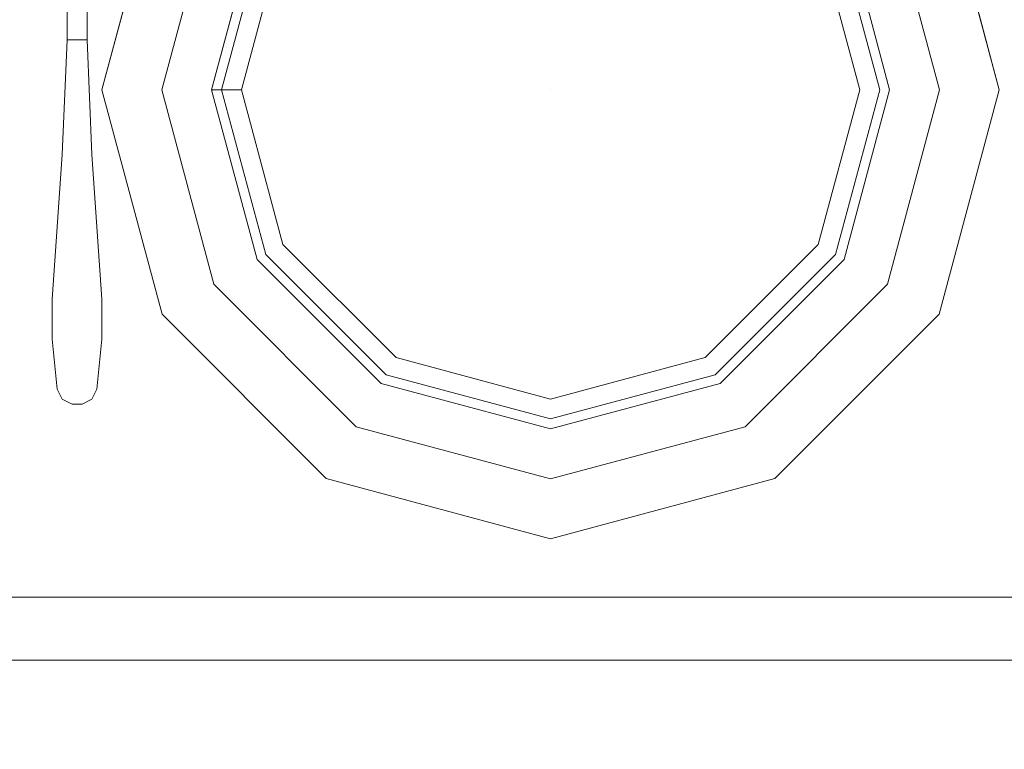
# Model space of a CAD drawing. Units: inches. Extents: x 375 to 1122, y 27 to 1069.
# Tile 86 of 155: x 719.12 to 731.28, y 845.63 to 854.63. Entities that reach past the tile are written whole.
import ezdxf

# ---------------------------------------------------------------- set-up
doc = ezdxf.new("R2010")
doc.units = ezdxf.units.IN
doc.layers.add('A-ANNO-DIMS', color=2, linetype='Continuous', lineweight=18)
doc.layers.add('Furniture', color=30, linetype='Continuous', lineweight=18)
doc.styles.get("Standard").update_dxf_attribs({"font": 'arial.ttf'})
doc.dimstyles.new('ISO-25', dxfattribs={"dimtxt": 12, "dimasz": 2.5, "dimexe": 1.5, "dimexo": 1.5, "dimtad": 1, "dimdec": 1, "dimlunit": 3, "dimtxsty": 'Standard', "dimblk": 'ARCHTICK', "dimcen": 2.5, "dimadec": 0, "dimazin": 0, "dimtfac": 1, "dimtdec": 1, "dimtmove": 0, "dimatfit": 3, "dimfxl": 1.5, "dimfxlon": 1, "dimarcsym": 0})

# ---------------------------------------------------------------- blocks, each defined once
blk = doc.blocks.new('A$C403C54AD')
for p, q in [((2.27071, 1.26108, -0.0006), (2.27071, 0.79569, -0.0006)), ((2.2901, 1.26108, -0.0006), (2.2901, 0.79569, -0.0006))]:
    blk.add_line(p, q)
at = {"linetype": 'ByBlock'}
for points, invisible_edges in [([(2.11411, 1.15687, -0.03783), (2.11411, 1.1384, -0.03783), (2.05409, 1.12232, -0.03783), (2.04485, 1.13831, -0.03783)], 5), ([(2.11411, 1.12301, -0.05168), (2.11411, 1.15687, -0.04244), (2.04485, 1.13831, -0.04244), (2.06178, 1.10899, -0.05168)], 5), ([(2.18338, 1.13831, -0.03783), (2.17414, 1.12232, -0.03783), (2.11411, 1.1384, -0.03783), (2.11411, 1.15687, -0.03783)], 5), ([(2.16645, 1.10899, -0.05168), (2.18338, 1.13831, -0.04244), (2.11411, 1.15687, -0.04244), (2.11411, 1.12301, -0.05168)], 5), ([(2.11411, 1.1384, -0.03783), (2.11411, 1.11993, -0.04398), (2.06332, 1.10632, -0.04398), (2.05409, 1.12232, -0.03783)], 5), ([(2.17414, 1.12232, -0.03783), (2.16491, 1.10632, -0.04398), (2.11411, 1.11993, -0.04398), (2.11411, 1.1384, -0.03783)], 5), ([(2.20476, 1.07068, -0.05168), (2.23408, 1.08761, -0.04244), (2.18338, 1.13831, -0.04244), (2.16645, 1.10899, -0.05168)], 5), ([(2.23408, 1.08761, -0.03783), (2.21809, 1.07837, -0.03783), (2.17414, 1.12232, -0.03783), (2.18338, 1.13831, -0.03783)], 5), ([(2.11411, 1.11377, -0.06091), (2.11411, 1.12301, -0.05168), (2.06178, 1.10899, -0.05168), (2.0664, 1.10099, -0.06091)], 5), ([(2.16183, 1.10099, -0.06091), (2.16645, 1.10899, -0.05168), (2.11411, 1.12301, -0.05168), (2.11411, 1.11377, -0.06091)], 5), ([(2.21809, 1.07837, -0.03783), (2.20209, 1.06914, -0.04398), (2.16491, 1.10632, -0.04398), (2.17414, 1.12232, -0.03783)], 5), ([(2.11411, 1.11993, -0.04398), (2.11411, 1.01834, -0.04398), (2.11411, 1.01834, -0.04398), (2.06332, 1.10632, -0.04398)], 5), ([(2.16491, 1.10632, -0.04398), (2.11411, 1.01834, -0.04398), (2.11411, 1.01834, -0.04398), (2.11411, 1.11993, -0.04398)], 5), ([(2.19676, 1.06606, -0.06091), (2.20476, 1.07068, -0.05168), (2.16645, 1.10899, -0.05168), (2.16183, 1.10099, -0.06091)], 5), ([(2.06332, 1.10632, -0.04398), (2.11411, 1.01834, -0.04398), (2.11411, 1.01834, -0.04398), (2.02614, 1.06914, -0.04398)], 5), ([(2.20209, 1.06914, -0.04398), (2.11411, 1.01834, -0.04398), (2.11411, 1.01834, -0.04398), (2.16491, 1.10632, -0.04398)], 5), ([(2.21878, 1.01834, -0.05168), (2.25264, 1.01834, -0.04244), (2.23408, 1.08761, -0.04244), (2.20476, 1.07068, -0.05168)], 5), ([(2.25264, 1.01834, -0.03783), (2.23417, 1.01834, -0.03783), (2.21809, 1.07837, -0.03783), (2.23408, 1.08761, -0.03783)], 5), ([(2.23417, 1.01834, -0.03783), (2.2157, 1.01834, -0.04398), (2.20209, 1.06914, -0.04398), (2.21809, 1.07837, -0.03783)], 5), ([(2.20954, 1.01834, -0.06091), (2.21878, 1.01834, -0.05168), (2.20476, 1.07068, -0.05168), (2.19676, 1.06606, -0.06091)], 5), ([(2.02614, 1.06914, -0.04398), (2.11411, 1.01834, -0.04398), (2.11411, 1.01834, -0.04398), (2.01253, 1.01834, -0.04398)], 5), ([(2.2157, 1.01834, -0.04398), (2.11411, 1.01834, -0.04398), (2.11411, 1.01834, -0.04398), (2.20209, 1.06914, -0.04398)], 5), ([(2.01253, 1.01834, -0.04398), (2.11411, 1.01834, -0.04398), (2.11411, 1.01834, -0.04398), (2.02614, 0.96755, -0.04398)], 5), ([(2.02614, 0.96755, -0.04398), (2.11411, 1.01834, -0.04398), (2.11411, 1.01834, -0.04398), (2.06332, 0.93037, -0.04398)], 5), ([(2.06332, 0.93037, -0.04398), (2.11411, 1.01834, -0.04398), (2.11411, 1.01834, -0.04398), (2.11411, 0.91676, -0.04398)], 5), ([(2.20209, 0.96755, -0.04398), (2.11411, 1.01834, -0.04398), (2.11411, 1.01834, -0.04398), (2.2157, 1.01834, -0.04398)], 5), ([(2.16491, 0.93037, -0.04398), (2.11411, 1.01834, -0.04398), (2.11411, 1.01834, -0.04398), (2.20209, 0.96755, -0.04398)], 5), ([(2.11411, 0.91676, -0.04398), (2.11411, 1.01834, -0.04398), (2.11411, 1.01834, -0.04398), (2.16491, 0.93037, -0.04398)], 5), ([(2.19676, 0.97063, -0.06091), (2.20476, 0.96601, -0.05168), (2.21878, 1.01834, -0.05168), (2.20954, 1.01834, -0.06091)], 5), ([(2.21809, 0.95832, -0.03783), (2.20209, 0.96755, -0.04398), (2.2157, 1.01834, -0.04398), (2.23417, 1.01834, -0.03783)], 5), ([(2.20476, 0.96601, -0.05168), (2.23408, 0.94908, -0.04244), (2.25264, 1.01834, -0.04244), (2.21878, 1.01834, -0.05168)], 5), ([(2.23408, 0.94908, -0.03783), (2.21809, 0.95832, -0.03783), (2.23417, 1.01834, -0.03783), (2.25264, 1.01834, -0.03783)], 5), ([(2.16183, 0.9357, -0.06091), (2.16645, 0.9277, -0.05168), (2.20476, 0.96601, -0.05168), (2.19676, 0.97063, -0.06091)], 5), ([(2.17414, 0.91437, -0.03783), (2.16491, 0.93037, -0.04398), (2.20209, 0.96755, -0.04398), (2.21809, 0.95832, -0.03783)], 5), ([(2.16645, 0.9277, -0.05168), (2.18338, 0.89838, -0.04244), (2.23408, 0.94908, -0.04244), (2.20476, 0.96601, -0.05168)], 5), ([(2.18338, 0.89838, -0.03783), (2.17414, 0.91437, -0.03783), (2.21809, 0.95832, -0.03783), (2.23408, 0.94908, -0.03783)], 5), ([(2.11411, 0.92291, -0.06091), (2.11411, 0.91368, -0.05168), (2.16645, 0.9277, -0.05168), (2.16183, 0.9357, -0.06091)], 4), ([(2.05409, 0.91437, -0.03783), (2.06332, 0.93037, -0.04398), (2.11411, 0.91676, -0.04398), (2.11411, 0.89829, -0.03783)], 5), ([(2.11411, 0.89829, -0.03783), (2.11411, 0.91676, -0.04398), (2.16491, 0.93037, -0.04398), (2.17414, 0.91437, -0.03783)], 5), ([(2.06178, 0.9277, -0.05168), (2.04485, 0.89838, -0.04244), (2.11411, 0.87982, -0.04244), (2.11411, 0.91368, -0.05168)], 5), ([(2.11411, 0.91368, -0.05168), (2.11411, 0.87982, -0.04244), (2.18338, 0.89838, -0.04244), (2.16645, 0.9277, -0.05168)], 5), ([(2.04485, 0.89838, -0.03783), (2.05409, 0.91437, -0.03783), (2.11411, 0.89829, -0.03783), (2.11411, 0.87982, -0.03783)], 5), ([(2.11411, 0.87982, -0.03783), (2.11411, 0.89829, -0.03783), (2.17414, 0.91437, -0.03783), (2.18338, 0.89838, -0.03783)], 5)]:
    blk.add_3dface(points, dxfattribs=dict(at, invisible_edges=invisible_edges))
for points in [[(2.11411, 1.15687, -0.04244), (2.11411, 1.15687, -0.03783), (2.04485, 1.13831, -0.03783), (2.04485, 1.13831, -0.04244)], [(2.18338, 1.13831, -0.04244), (2.18338, 1.13831, -0.03783), (2.11411, 1.15687, -0.03783), (2.11411, 1.15687, -0.04244)], [(2.23408, 1.08761, -0.04244), (2.23408, 1.08761, -0.03783), (2.18338, 1.13831, -0.03783), (2.18338, 1.13831, -0.04244)], [(2.25264, 1.01834, -0.04244), (2.25264, 1.01834, -0.03783), (2.23408, 1.08761, -0.03783), (2.23408, 1.08761, -0.04244)], [(2.23408, 0.94908, -0.04244), (2.23408, 0.94908, -0.03783), (2.25264, 1.01834, -0.03783), (2.25264, 1.01834, -0.04244)], [(2.18338, 0.89838, -0.04244), (2.18338, 0.89838, -0.03783), (2.23408, 0.94908, -0.03783), (2.23408, 0.94908, -0.04244)], [(2.0664, 0.9357, -0.06091), (2.06178, 0.9277, -0.05168), (2.11411, 0.91368, -0.05168), (2.11411, 0.92291, -0.06091)], [(2.04485, 0.89838, -0.04244), (2.04485, 0.89838, -0.03783), (2.11411, 0.87982, -0.03783), (2.11411, 0.87982, -0.04244)], [(2.11411, 0.87982, -0.04244), (2.11411, 0.87982, -0.03783), (2.18338, 0.89838, -0.03783), (2.18338, 0.89838, -0.04244)]]:
    blk.add_3dface(points, dxfattribs=at)
for points, invisible_edges in [([(2.17876, 0.86443, -0.04825), (2.17876, 0.87982, -0.04825), (2.13412, 0.87674, -0.04587), (2.13412, 0.8675, -0.04587)], 5), ([(2.17876, 0.86443, -0.05289), (2.17876, 0.87982, -0.05289), (2.13412, 0.87674, -0.04895), (2.13412, 0.8675, -0.04895)], 5), ([(2.17876, 0.87982, -0.05289), (2.17876, 0.87982, -0.04825), (2.13412, 0.87674, -0.04587), (2.13412, 0.87674, -0.04895)], 4), ([(2.19107, 0.87982, -0.04858), (2.19107, 0.86443, -0.04858), (2.17876, 0.86443, -0.04825), (2.17876, 0.87982, -0.04825)], 5), ([(2.19107, 0.87982, -0.05321), (2.19107, 0.86443, -0.05321), (2.17876, 0.86443, -0.05289), (2.17876, 0.87982, -0.05289)], 5), ([(2.20647, 0.86596, -0.04855), (2.20647, 0.87828, -0.04855), (2.19107, 0.87982, -0.04858), (2.19107, 0.86443, -0.04858)], 5), ([(2.20647, 0.86596, -0.05318), (2.20647, 0.87828, -0.05318), (2.19107, 0.87982, -0.05321), (2.19107, 0.86443, -0.05321)], 5), ([(2.13412, 0.87674, -0.04587), (2.13412, 0.8675, -0.04587), (2.09872, 0.86904, -0.04296), (2.09872, 0.8752, -0.04296)], 1), ([(2.13412, 0.87674, -0.04587), (2.13412, 0.87674, -0.04895), (2.09872, 0.8752, -0.04555), (2.09872, 0.8752, -0.04296)], 5), ([(2.13412, 0.87674, -0.04895), (2.13412, 0.8675, -0.04895), (2.09872, 0.86904, -0.04555), (2.09872, 0.8752, -0.04555)], 1), ([(2.20954, 0.87674, -0.0483), (2.20954, 0.8675, -0.0483), (2.20647, 0.86596, -0.04855), (2.20647, 0.87828, -0.04855)], 5), ([(2.20954, 0.87674, -0.05294), (2.20954, 0.8675, -0.05294), (2.20647, 0.86596, -0.05318), (2.20647, 0.87828, -0.05318)], 5), ([(2.21108, 0.87058, -0.04847), (2.21108, 0.87366, -0.04847), (2.20954, 0.87674, -0.0483), (2.20954, 0.8675, -0.0483)], 4), ([(2.21108, 0.87058, -0.0526), (2.21108, 0.87366, -0.0526), (2.20954, 0.87674, -0.05294), (2.20954, 0.8675, -0.05294)], 4), ([(2.09872, 0.8752, -0.04555), (2.09872, 0.8752, -0.04296), (2.08795, 0.8752, -0.04504), (2.08795, 0.8752, -0.04763)], 5), ([(2.08795, 0.86904, -0.04763), (2.08795, 0.86904, -0.04504), (2.09872, 0.86904, -0.04296), (2.09872, 0.86904, -0.04555)], 5), ([(2.09872, 0.86904, -0.04296), (2.09872, 0.86904, -0.04555), (2.13412, 0.8675, -0.04895), (2.13412, 0.8675, -0.04587)], 5), ([(2.13412, 0.8675, -0.04895), (2.13412, 0.8675, -0.04587), (2.17876, 0.86443, -0.04825), (2.17876, 0.86443, -0.05289)], 1)]:
    blk.add_3dface(points, dxfattribs=dict(invisible_edges=invisible_edges))
for points in [[(2.19107, 0.87982, -0.04858), (2.19107, 0.87982, -0.05321), (2.17876, 0.87982, -0.05289), (2.17876, 0.87982, -0.04825)], [(2.20647, 0.87828, -0.05318), (2.20647, 0.87828, -0.04855), (2.19107, 0.87982, -0.04858), (2.19107, 0.87982, -0.05321)], [(2.20954, 0.87674, -0.0483), (2.20954, 0.87674, -0.05294), (2.20647, 0.87828, -0.05318), (2.20647, 0.87828, -0.04855)], [(2.21108, 0.87366, -0.0526), (2.21108, 0.87366, -0.04847), (2.20954, 0.87674, -0.0483), (2.20954, 0.87674, -0.05294)], [(2.09872, 0.86904, -0.04296), (2.09872, 0.8752, -0.04296), (2.08795, 0.8752, -0.04504), (2.08795, 0.86904, -0.04504)], [(2.09872, 0.86904, -0.04555), (2.09872, 0.8752, -0.04555), (2.08795, 0.8752, -0.04763), (2.08795, 0.86904, -0.04763)], [(2.21108, 0.87058, -0.04847), (2.21108, 0.87058, -0.0526), (2.21108, 0.87366, -0.0526), (2.21108, 0.87366, -0.04847)], [(2.20954, 0.8675, -0.05294), (2.20954, 0.8675, -0.0483), (2.21108, 0.87058, -0.04847), (2.21108, 0.87058, -0.0526)], [(2.20647, 0.86596, -0.04855), (2.20647, 0.86596, -0.05318), (2.20954, 0.8675, -0.05294), (2.20954, 0.8675, -0.0483)], [(2.17876, 0.86443, -0.04825), (2.17876, 0.86443, -0.05289), (2.19107, 0.86443, -0.05321), (2.19107, 0.86443, -0.04858)], [(2.19107, 0.86443, -0.05321), (2.19107, 0.86443, -0.04858), (2.20647, 0.86596, -0.04855), (2.20647, 0.86596, -0.05318)]]:
    blk.add_3dface(points)
blk = doc.blocks.new('_ArchTick')
at = {"color": 0, "linetype": 'ByBlock', "const_width": 0.15}
blk.add_lwpolyline([(-0.5, -0.5), (0.5, 0.5)], dxfattribs=at)
blk = doc.blocks.new('*D85')
at = {"layer": 'A-ANNO-DIMS', "color": 0, "lineweight": -2, "transparency": 16777216}
for p, q in [((401.507, 868.528), (398.507, 868.528)), ((400.007, 814.528), (400.007, 868.528)), ((401.507, 814.528), (398.507, 814.528))]:
    blk.add_line(p, q, dxfattribs=at)
at = {"layer": 'Defpoints', "color": 0, "transparency": 16777216}
for p in [(400.007, 868.528), (845.007, 868.528), (845.007, 814.528)]:
    blk.add_point(p, dxfattribs=at)
at = {"layer": 'A-ANNO-DIMS', "color": 0, "lineweight": -2, "transparency": 16777216, "xscale": 2.5, "yscale": 2.5, "zscale": 2.5}
for p, rotation in [((400.007, 868.528), 90), ((400.007, 814.528), 270)]:
    blk.add_blockref('_ArchTick', p, dxfattribs=dict(at, rotation=rotation))
at = {"layer": 'A-ANNO-DIMS', "color": 0, "transparency": 16777216, "insert": (393.255, 841.528), "char_height": 12, "attachment_point": 5, "rotation": 90}
blk.add_mtext('4\'-6"', dxfattribs=at)
blk = doc.blocks.new('*D88')
at = {"layer": 'A-ANNO-DIMS', "color": 0, "lineweight": -2, "transparency": 16777216}
for p, q in [((731.007, 1052.528), (731.007, 1055.528)), ((854.007, 1052.528), (854.007, 1055.528)), ((731.007, 1054.028), (854.007, 1054.028))]:
    blk.add_line(p, q, dxfattribs=at)
at = {"layer": 'Defpoints', "color": 0, "transparency": 16777216}
for p in [(854.007, 1054.028), (731.007, 502.528), (854.007, 502.528)]:
    blk.add_point(p, dxfattribs=at)
at = {"layer": 'A-ANNO-DIMS', "color": 0, "lineweight": -2, "transparency": 16777216, "xscale": 2.5, "yscale": 2.5, "zscale": 2.5, "rotation": 180}
blk.add_blockref('_ArchTick', (731.007, 1054.028), dxfattribs=at)
at = {"layer": 'A-ANNO-DIMS', "color": 0, "lineweight": -2, "transparency": 16777216, "xscale": 2.5, "yscale": 2.5, "zscale": 2.5}
blk.add_blockref('_ArchTick', (854.007, 1054.028), dxfattribs=at)
at = {"layer": 'A-ANNO-DIMS', "color": 0, "transparency": 16777216, "insert": (792.507, 1060.784), "char_height": 12, "attachment_point": 5}
blk.add_mtext('10\'-3"', dxfattribs=at)
blk = doc.blocks.new('*D91')
at = {"layer": 'A-ANNO-DIMS', "color": 0, "lineweight": -2, "transparency": 16777216}
for p, q in [((728.007, 1052.528), (728.007, 1055.528)), ((788.007, 1052.528), (788.007, 1055.528)), ((728.007, 1054.028), (788.007, 1054.028))]:
    blk.add_line(p, q, dxfattribs=at)
at = {"layer": 'Defpoints', "color": 0, "transparency": 16777216}
for p in [(788.007, 1054.028), (728.007, 774.028), (788.007, 774.028)]:
    blk.add_point(p, dxfattribs=at)
at = {"layer": 'A-ANNO-DIMS', "color": 0, "lineweight": -2, "transparency": 16777216, "xscale": 2.5, "yscale": 2.5, "zscale": 2.5, "rotation": 180}
blk.add_blockref('_ArchTick', (728.007, 1054.028), dxfattribs=at)
at = {"layer": 'A-ANNO-DIMS', "color": 0, "lineweight": -2, "transparency": 16777216, "xscale": 2.5, "yscale": 2.5, "zscale": 2.5}
blk.add_blockref('_ArchTick', (788.007, 1054.028), dxfattribs=at)
at = {"layer": 'A-ANNO-DIMS', "color": 0, "transparency": 16777216, "insert": (758.007, 1060.78), "char_height": 12, "attachment_point": 5}
blk.add_mtext('5\'-0"', dxfattribs=at)

msp = doc.modelspace()

# ---------------------------------------------------------------- block references
at = {"layer": 'Furniture', "xscale": 39.9918517141215, "yscale": 39.9918517141215, "zscale": 39.9918517141215, "rotation": 270}
msp.add_blockref('A$C403C54AD', (684.955, 938.316, 0.024), dxfattribs=at)

# ---------------------------------------------------------------- dimensions: what is measured, and where the dimension line sits
at = {"layer": 'A-ANNO-DIMS'}
for base, p1, p2, picture, middle in [((788.007, 1054.028), (728.007, 774.028), (788.007, 774.028), '*D91', (758.007, 1060.78)), ((854.007, 1054.028), (731.007, 502.528), (854.007, 502.528), '*D88', (792.507, 1060.784))]:
    dim = msp.add_linear_dim(base=base, p1=p1, p2=p2, dimstyle='ISO-25', override={"dimdec": 1, "dimlfac": 1, "dimrnd": 0, "dimzin": 1, "dimdsep": 46, "dimlunit": 4, "dimfrac": 2}, dxfattribs=at)
    dim.commit()
    dim.dimension.update_dxf_attribs({"geometry": picture, "text_midpoint": middle})
dim = msp.add_linear_dim(base=(400.007, 868.528), p1=(845.007, 814.528), p2=(845.007, 868.528), angle=90, dimstyle='ISO-25', override={"dimdec": 1, "dimlfac": 1, "dimrnd": 0, "dimzin": 1, "dimdsep": 46, "dimlunit": 4, "dimfrac": 2}, dxfattribs=at)
dim.commit()
dim.dimension.update_dxf_attribs({"geometry": '*D85', "text_midpoint": (393.255, 841.528)})

doc.saveas('drawing.dxf')
